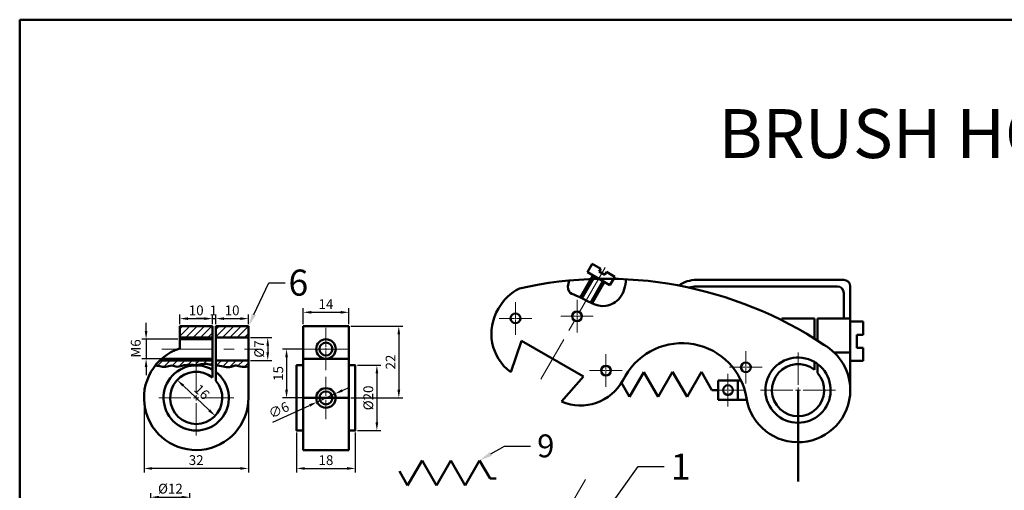
# Model space of a CAD drawing. Units: millimetres. Extents: x 77 to 718, y -35 to 313.
# Tile 3 of 7: x 77 to 379, y 169 to 313. Entities that reach past the tile are written whole.
import ezdxf
from ezdxf import colors
from ezdxf.entities.mleader import LeaderData, LeaderLine
from ezdxf.math import Vec2, Vec3

# ---------------------------------------------------------------- set-up
doc = ezdxf.new("R2010")
doc.units = ezdxf.units.MM
doc.header["$LTSCALE"] = 0.5
doc.linetypes.add('CENTER', pattern=[50.800000000000004, 31.75, -6.349999999999999, 6.349999999999999, -6.349999999999999])
for name, color, linetype, lineweight in [('M-CNTR', 1, 'CENTER', 18), ('M-DIMS', 2, 'Continuous', 25), ('M-HATC', 8, 'Continuous', 18), ('M-OUTL', 7, 'Continuous', 50), ('M-TEXT', 3, 'Continuous', 25)]:
    doc.layers.add(name, color=color, linetype=linetype, lineweight=lineweight)
doc.styles.get("Standard").update_dxf_attribs({"font": 'arial.ttf'})
doc.dimstyles.new('ISO-25', dxfattribs={"dimtxt": 3, "dimasz": 2.5, "dimexe": 1.25, "dimexo": 0.625, "dimtad": 1, "dimtxsty": 'Standard', "dimcen": 2.5, "dimadec": 0, "dimazin": 0, "dimtfac": 1, "dimtmove": 0, "dimatfit": 3, "dimfxl": 1, "dimarcsym": 0})
pattern_1 = [(45, (-102.577664864981, 114.7341887866325), (-1.122532015133644, 1.122532015133644), [])]

# ---------------------------------------------------------------- blocks, each defined once
blk = doc.blocks.new('*D2')
at = {"layer": 'Defpoints', "color": 0, "transparency": 16777216}
for p in [(129.6092219175839, 166.4736375259157), (117.6092219175839, 162.0709279252485), (129.6092219175839, 162.0709279252485)]:
    blk.add_point(p, dxfattribs=at)
at = {"layer": 'M-DIMS', "color": 0, "lineweight": -2, "transparency": 16777216}
for p, q in [((117.6092219175839, 162.6959279252485), (117.6092219175839, 167.7236375259157)), ((120.1092219175839, 166.4736375259157), (127.1092219175839, 166.4736375259157)), ((129.6092219175839, 162.6959279252485), (129.6092219175839, 167.7236375259157))]:
    blk.add_line(p, q, dxfattribs=at)
at = {"layer": 'M-DIMS', "color": 0, "transparency": 16777216}
for points in [[(120.1092219175839, 166.8903041925824), (120.1092219175839, 166.0569708592491), (117.6092219175839, 166.4736375259157)], [(127.1092219175839, 166.8903041925824), (127.1092219175839, 166.0569708592491), (129.6092219175839, 166.4736375259157)]]:
    blk.add_solid(points, dxfattribs=at)
at = {"layer": 'M-DIMS', "color": 0, "transparency": 16777216, "insert": (123.6092219175839, 168.7142582626142), "char_height": 3, "attachment_point": 5}
blk.add_mtext('%%C12', dxfattribs=at)
blk = doc.blocks.new('*U32')
at = {"layer": 'M-CNTR', "color": 0, "transparency": 16777216}
for p, q in [((0, 1.6), (0, 11.5)), ((-11.5, 0), (-1.599999999999999, 0)), ((1.6, 0), (11.5, 0)), ((0, -11.5), (0, -1.599999999999999))]:
    blk.add_line(p, q, dxfattribs=at)
at = {"layer": 'M-CNTR', "color": 0, "linetype": 'Continuous', "transparency": 16777216}
for p, q in [((-0.8, 0), (0.8, 0)), ((0, -0.8), (0, 0.8))]:
    blk.add_line(p, q, dxfattribs=at)
blk = doc.blocks.new('*U33')
at = {"layer": 'M-CNTR', "color": 0, "transparency": 16777216}
for p, q in [((0, 1.6), (0, 11.5)), ((-11.5, 0), (-1.599999999999999, 0)), ((1.6, 0), (11.5, 0)), ((0, -11.5), (0, -1.599999999999999))]:
    blk.add_line(p, q, dxfattribs=at)
at = {"layer": 'M-CNTR', "color": 0, "linetype": 'Continuous', "transparency": 16777216}
for p, q in [((-0.8, 0), (0.8, 0)), ((0, -0.8), (0, 0.8))]:
    blk.add_line(p, q, dxfattribs=at)
blk = doc.blocks.new('*U34')
at = {"layer": 'M-CNTR', "color": 0, "transparency": 16777216}
for p, q in [((0, 0.6000000000000001), (0, 6.5)), ((-6.5, 0), (-0.5999999999999996, 0)), ((0.6000000000000001, 0), (6.5, 0)), ((0, -6.5), (0, -0.5999999999999996))]:
    blk.add_line(p, q, dxfattribs=at)
at = {"layer": 'M-CNTR', "color": 0, "linetype": 'Continuous', "transparency": 16777216}
for p, q in [((-0.3, 0), (0.3, 0)), ((0, -0.3), (0, 0.3))]:
    blk.add_line(p, q, dxfattribs=at)
blk = doc.blocks.new('*U35')
at = {"layer": 'M-CNTR', "color": 0, "transparency": 16777216}
for p, q in [((0, 0.6000000000000001), (0, 6.5)), ((-6.5, 0), (-0.5999999999999996, 0)), ((0.6000000000000001, 0), (6.5, 0)), ((0, -6.5), (0, -0.5999999999999996))]:
    blk.add_line(p, q, dxfattribs=at)
at = {"layer": 'M-CNTR', "color": 0, "linetype": 'Continuous', "transparency": 16777216}
for p, q in [((-0.3, 0), (0.3, 0)), ((0, -0.3), (0, 0.3))]:
    blk.add_line(p, q, dxfattribs=at)
blk = doc.blocks.new('*D36')
at = {"layer": 'Defpoints', "color": 0, "transparency": 16777216}
for p in [(178.2884430352653, 223.1732257711527), (164.2884430352653, 218.9185971032211), (178.2884430352653, 218.9185971032211)]:
    blk.add_point(p, dxfattribs=at)
at = {"layer": 'M-DIMS', "color": 0, "lineweight": -2, "transparency": 16777216}
for p, q in [((164.2884430352653, 219.5435971032211), (164.2884430352653, 224.4232257711527)), ((178.2884430352653, 219.5435971032211), (178.2884430352653, 224.4232257711527)), ((166.7884430352653, 223.1732257711527), (175.7884430352653, 223.1732257711527))]:
    blk.add_line(p, q, dxfattribs=at)
at = {"layer": 'M-DIMS', "color": 0, "transparency": 16777216}
for points in [[(166.7884430352653, 223.5898924378194), (166.7884430352653, 222.7565591044861), (164.2884430352653, 223.1732257711527)], [(175.7884430352653, 223.5898924378194), (175.7884430352653, 222.7565591044861), (178.2884430352653, 223.1732257711527)]]:
    blk.add_solid(points, dxfattribs=at)
at = {"layer": 'M-DIMS', "color": 0, "transparency": 16777216, "insert": (171.2884430352653, 225.3043649253137), "char_height": 3, "attachment_point": 5}
blk.add_mtext('14', dxfattribs=at)
blk = doc.blocks.new('*D37')
at = {"layer": 'Defpoints', "color": 0, "transparency": 16777216}
for p in [(178.2884430352654, 218.9185971032212), (178.2884430352654, 196.9185971032212), (193.6241074583753, 196.9185971032212)]:
    blk.add_point(p, dxfattribs=at)
at = {"layer": 'M-DIMS', "color": 0, "lineweight": -2, "transparency": 16777216}
for p, q in [((178.9134430352654, 218.9185971032212), (194.8741074583753, 218.9185971032213)), ((193.6241074583753, 216.4185971032212), (193.6241074583753, 199.4185971032212)), ((178.9134430352654, 196.9185971032212), (194.8741074583753, 196.9185971032212))]:
    blk.add_line(p, q, dxfattribs=at)
at = {"layer": 'M-DIMS', "color": 0, "transparency": 16777216}
for points in [[(193.2074407917086, 216.4185971032212), (194.0407741250419, 216.4185971032212), (193.6241074583753, 218.9185971032213)], [(193.2074407917086, 199.4185971032212), (194.0407741250419, 199.4185971032212), (193.6241074583753, 196.9185971032212)]]:
    blk.add_solid(points, dxfattribs=at)
at = {"layer": 'M-DIMS', "color": 0, "transparency": 16777216, "insert": (191.4929683042143, 207.918597103221), "char_height": 3, "attachment_point": 5, "rotation": 90}
blk.add_mtext('22', dxfattribs=at)
blk = doc.blocks.new('*D38')
at = {"layer": 'Defpoints', "color": 0, "transparency": 16777216}
for p in [(180.2884430352653, 206.9185971032212), (180.2884430352653, 186.9185971032211), (186.8937752468204, 186.9185971032211)]:
    blk.add_point(p, dxfattribs=at)
at = {"layer": 'M-DIMS', "color": 0, "lineweight": -2, "transparency": 16777216}
for p, q in [((180.9134430352653, 206.9185971032212), (188.1437752468203, 206.9185971032212)), ((186.8937752468203, 204.4185971032212), (186.8937752468204, 189.4185971032211)), ((180.9134430352653, 186.9185971032211), (188.1437752468204, 186.9185971032211))]:
    blk.add_line(p, q, dxfattribs=at)
at = {"layer": 'M-DIMS', "color": 0, "transparency": 16777216}
for points in [[(186.4771085801537, 204.4185971032212), (187.310441913487, 204.4185971032212), (186.8937752468203, 206.9185971032212)], [(186.4771085801537, 189.4185971032211), (187.310441913487, 189.4185971032211), (186.8937752468204, 186.9185971032211)]]:
    blk.add_solid(points, dxfattribs=at)
at = {"layer": 'M-DIMS', "color": 0, "transparency": 16777216, "insert": (184.6531545101218, 196.9185971032211), "char_height": 3, "attachment_point": 5, "rotation": 90}
blk.add_mtext('%%C20', dxfattribs=at)
blk = doc.blocks.new('*D39')
at = {"layer": 'Defpoints', "color": 0, "transparency": 16777216}
for p in [(136.5191626098565, 221.2361377014674), (126.5191626098565, 218.9185971032211), (136.5191626098565, 218.9185971032211)]:
    blk.add_point(p, dxfattribs=at)
at = {"layer": 'M-DIMS', "color": 0, "lineweight": -2, "transparency": 16777216}
for p, q in [((126.5191626098565, 219.5435971032211), (126.5191626098565, 222.4861377014674)), ((129.0191626098565, 221.2361377014674), (134.0191626098565, 221.2361377014674)), ((136.5191626098565, 219.5435971032211), (136.5191626098565, 222.4861377014674))]:
    blk.add_line(p, q, dxfattribs=at)
at = {"layer": 'M-DIMS', "color": 0, "transparency": 16777216}
for points in [[(129.0191626098565, 221.6528043681341), (129.0191626098565, 220.8194710348007), (126.5191626098565, 221.2361377014674)], [(134.0191626098565, 221.6528043681341), (134.0191626098565, 220.8194710348007), (136.5191626098565, 221.2361377014674)]]:
    blk.add_solid(points, dxfattribs=at)
at = {"layer": 'M-DIMS', "color": 0, "transparency": 16777216, "insert": (131.5191626098565, 223.3928566646325), "char_height": 3, "attachment_point": 5}
blk.add_mtext('10', dxfattribs=at)
blk = doc.blocks.new('*D40')
at = {"layer": 'Defpoints', "color": 0, "transparency": 16777216}
for p in [(137.5191626098565, 221.2361377014674), (136.5191626098565, 218.9185971032211), (137.5191626098565, 218.9185971032211)]:
    blk.add_point(p, dxfattribs=at)
at = {"layer": 'M-DIMS', "color": 0, "lineweight": -2, "transparency": 16777216}
for p, q in [((134.0191626098565, 221.2361377014674), (131.5191626098565, 221.2361377014674)), ((136.5191626098565, 219.5435971032211), (136.5191626098565, 222.4861377014674)), ((136.5191626098565, 221.2361377014674), (137.5191626098565, 221.2361377014674)), ((137.5191626098565, 219.5435971032211), (137.5191626098565, 222.4861377014674)), ((140.0191626098565, 221.2361377014674), (142.5191626098565, 221.2361377014674))]:
    blk.add_line(p, q, dxfattribs=at)
at = {"layer": 'M-DIMS', "color": 0, "transparency": 16777216}
for points in [[(134.0191626098565, 221.6528043681341), (134.0191626098565, 220.8194710348007), (136.5191626098565, 221.2361377014674)], [(140.0191626098565, 221.6528043681341), (140.0191626098565, 220.8194710348007), (137.5191626098565, 221.2361377014674)]]:
    blk.add_solid(points, dxfattribs=at)
at = {"layer": 'M-DIMS', "color": 0, "transparency": 16777216, "insert": (136.7740427016174, 223.3672768556283), "char_height": 3, "attachment_point": 5}
blk.add_mtext('1', dxfattribs=at)
blk = doc.blocks.new('*D41')
at = {"layer": 'Defpoints', "color": 0, "transparency": 16777216}
for p in [(147.5191626098565, 221.2361377014674), (137.5191626098565, 218.9185971032211), (147.5191626098565, 218.9185971032211)]:
    blk.add_point(p, dxfattribs=at)
at = {"layer": 'M-DIMS', "color": 0, "lineweight": -2, "transparency": 16777216}
for p, q in [((137.5191626098565, 219.5435971032211), (137.5191626098565, 222.4861377014674)), ((140.0191626098565, 221.2361377014674), (145.0191626098565, 221.2361377014674)), ((147.5191626098565, 219.5435971032211), (147.5191626098565, 222.4861377014674))]:
    blk.add_line(p, q, dxfattribs=at)
at = {"layer": 'M-DIMS', "color": 0, "transparency": 16777216}
for points in [[(140.0191626098565, 221.6528043681341), (140.0191626098565, 220.8194710348007), (137.5191626098565, 221.2361377014674)], [(145.0191626098565, 221.6528043681341), (145.0191626098565, 220.8194710348007), (147.5191626098565, 221.2361377014674)]]:
    blk.add_solid(points, dxfattribs=at)
at = {"layer": 'M-DIMS', "color": 0, "transparency": 16777216, "insert": (142.5191626098565, 223.3928566646325), "char_height": 3, "attachment_point": 5}
blk.add_mtext('10', dxfattribs=at)
blk = doc.blocks.new('*D42')
at = {"layer": 'Defpoints', "color": 0, "transparency": 16777216}
for p in [(147.5191626098566, 215.4185971032212), (147.5191626098566, 208.4185971032212), (153.4383000049706, 208.4185971032212)]:
    blk.add_point(p, dxfattribs=at)
at = {"layer": 'M-DIMS', "color": 0, "lineweight": -2, "transparency": 16777216}
for p, q in [((148.1441626098566, 215.4185971032212), (154.6883000049706, 215.4185971032212)), ((153.4383000049706, 212.9185971032212), (153.4383000049706, 210.9185971032212)), ((148.1441626098566, 208.4185971032212), (154.6883000049706, 208.4185971032212))]:
    blk.add_line(p, q, dxfattribs=at)
at = {"layer": 'M-DIMS', "color": 0, "transparency": 16777216}
for points in [[(153.0216333383039, 212.9185971032212), (153.8549666716372, 212.9185971032212), (153.4383000049706, 215.4185971032212)], [(153.0216333383039, 210.9185971032212), (153.8549666716372, 210.9185971032212), (153.4383000049706, 208.4185971032212)]]:
    blk.add_solid(points, dxfattribs=at)
at = {"layer": 'M-DIMS', "color": 0, "transparency": 16777216, "insert": (151.1976792682721, 211.9185971032211), "char_height": 3, "attachment_point": 5, "rotation": 90}
blk.add_mtext('%%C7', dxfattribs=at)
blk = doc.blocks.new('*D43')
at = {"layer": 'Defpoints', "color": 0, "transparency": 16777216}
for p in [(126.5191626098566, 214.9185971032212), (116.1550390454235, 208.9185971032212), (126.5191626098566, 208.9185971032212)]:
    blk.add_point(p, dxfattribs=at)
at = {"layer": 'M-DIMS', "color": 0, "lineweight": -2, "transparency": 16777216}
for p, q in [((116.1550390454235, 217.4185971032212), (116.1550390454235, 219.9185971032212)), ((125.8941626098565, 214.9185971032212), (114.9050390454235, 214.9185971032212)), ((116.1550390454235, 214.9185971032212), (116.1550390454235, 208.9185971032212)), ((125.8941626098565, 208.9185971032212), (114.9050390454235, 208.9185971032212)), ((116.1550390454235, 206.4185971032212), (116.1550390454235, 203.9185971032212))]:
    blk.add_line(p, q, dxfattribs=at)
at = {"layer": 'M-DIMS', "color": 0, "transparency": 16777216}
for points in [[(115.7383723787568, 217.4185971032212), (116.5717057120902, 217.4185971032212), (116.1550390454235, 214.9185971032212)], [(115.7383723787568, 206.4185971032212), (116.5717057120902, 206.4185971032212), (116.1550390454235, 208.9185971032212)]]:
    blk.add_solid(points, dxfattribs=at)
at = {"layer": 'M-DIMS', "color": 0, "transparency": 16777216, "insert": (113.3727995653948, 212.0977955691644), "char_height": 3, "attachment_point": 5, "rotation": 90}
blk.add_mtext('M6', dxfattribs=at)
blk = doc.blocks.new('*D44')
at = {"layer": 'Defpoints', "color": 0, "transparency": 16777216}
for p in [(125.713031027325, 202.4221265204524), (137.3252941923879, 191.4150676859897), (137.325294192388, 191.4150676859898)]:
    blk.add_point(p, dxfattribs=at)
at = {"layer": 'M-DIMS', "color": 0, "lineweight": -2, "transparency": 16777216}
for p, q in [((126.1429942630462, 202.8757305503377), (126.5729574987675, 203.329334580223)), ((127.5274471468661, 200.7022735775677), (135.5108780728469, 193.1349206288746)), ((137.7552574281092, 191.868671715875), (138.1852206638304, 192.3222757457603))]:
    blk.add_line(p, q, dxfattribs=at)
at = {"layer": 'M-DIMS', "color": 0, "transparency": 16777216}
for points in [[(127.8140893040136, 201.0046762641578), (127.2408049897187, 200.3998708909775), (125.713031027325, 202.4221265204524)], [(135.7975202299944, 193.4373233154648), (135.2242359156994, 192.8325179422844), (137.325294192388, 191.4150676859898)]]:
    blk.add_solid(points, dxfattribs=at)
at = {"layer": 'M-DIMS', "color": 0, "transparency": 16777216, "insert": (133.0028583921665, 198.4838713640558), "char_height": 3, "attachment_point": 5, "rotation": 316.5326446484607}
blk.add_mtext('16', dxfattribs=at)
blk = doc.blocks.new('*D45')
at = {"layer": 'Defpoints', "color": 0, "transparency": 16777216}
for p in [(115.5191626098565, 196.918597103221), (147.5191626098565, 196.918597103221), (115.5191626098565, 175.3007429935038)]:
    blk.add_point(p, dxfattribs=at)
at = {"layer": 'M-DIMS', "color": 0, "lineweight": -2, "transparency": 16777216}
for p, q in [((115.5191626098565, 196.2935971032211), (115.5191626098565, 174.0507429935038)), ((147.5191626098565, 196.2935971032211), (147.5191626098565, 174.0507429935038)), ((145.0191626098565, 175.3007429935038), (118.0191626098565, 175.3007429935038))]:
    blk.add_line(p, q, dxfattribs=at)
at = {"layer": 'M-DIMS', "color": 0, "transparency": 16777216}
for points in [[(118.0191626098565, 175.7174096601705), (118.0191626098565, 174.8840763268372), (115.5191626098565, 175.3007429935038)], [(145.0191626098565, 175.7174096601705), (145.0191626098565, 174.8840763268372), (147.5191626098565, 175.3007429935038)]]:
    blk.add_solid(points, dxfattribs=at)
at = {"layer": 'M-DIMS', "color": 0, "transparency": 16777216, "insert": (131.5191626098565, 177.458485149029), "char_height": 3, "attachment_point": 5}
blk.add_mtext('32', dxfattribs=at)
blk = doc.blocks.new('*D46')
at = {"layer": 'Defpoints', "color": 0, "transparency": 16777216}
for p in [(162.2884430352654, 186.9185971032211), (180.2884430352653, 186.9185971032211), (180.2884430352653, 175.3007429935038)]:
    blk.add_point(p, dxfattribs=at)
at = {"layer": 'M-DIMS', "color": 0, "lineweight": -2, "transparency": 16777216}
for p, q in [((162.2884430352654, 186.2935971032211), (162.2884430352654, 174.0507429935038)), ((180.2884430352653, 186.2935971032211), (180.2884430352653, 174.0507429935038)), ((164.7884430352654, 175.3007429935038), (177.7884430352653, 175.3007429935038))]:
    blk.add_line(p, q, dxfattribs=at)
at = {"layer": 'M-DIMS', "color": 0, "transparency": 16777216}
for points in [[(164.7884430352654, 175.7174096601705), (164.7884430352654, 174.8840763268372), (162.2884430352654, 175.3007429935038)], [(177.7884430352653, 175.7174096601705), (177.7884430352653, 174.8840763268372), (180.2884430352653, 175.3007429935038)]]:
    blk.add_solid(points, dxfattribs=at)
at = {"layer": 'M-DIMS', "color": 0, "transparency": 16777216, "insert": (171.2884430352653, 177.4574619566689), "char_height": 3, "attachment_point": 5}
blk.add_mtext('18', dxfattribs=at)
blk = doc.blocks.new('*D47')
at = {"layer": 'Defpoints', "color": 0, "transparency": 16777216}
for p in [(164.7884430352654, 211.9185971032212), (159.2157581517809, 196.9185971032212), (164.7884430352654, 196.9185971032212)]:
    blk.add_point(p, dxfattribs=at)
at = {"layer": 'M-DIMS', "color": 0, "lineweight": -2, "transparency": 16777216}
for p, q in [((164.1634430352654, 211.9185971032212), (157.9657581517809, 211.9185971032212)), ((159.2157581517809, 209.4185971032212), (159.2157581517809, 199.4185971032212)), ((164.1634430352654, 196.9185971032212), (157.9657581517809, 196.9185971032212))]:
    blk.add_line(p, q, dxfattribs=at)
at = {"layer": 'M-DIMS', "color": 0, "transparency": 16777216}
for points in [[(158.7990914851142, 209.4185971032212), (159.6324248184475, 209.4185971032212), (159.2157581517809, 211.9185971032212)], [(158.7990914851142, 199.4185971032212), (159.6324248184475, 199.4185971032212), (159.2157581517809, 196.9185971032212)]]:
    blk.add_solid(points, dxfattribs=at)
at = {"layer": 'M-DIMS', "color": 0, "transparency": 16777216, "insert": (157.0590391886158, 204.4185971032211), "char_height": 3, "attachment_point": 5, "rotation": 90}
blk.add_mtext('15', dxfattribs=at)
blk = doc.blocks.new('*D48')
at = {"layer": 'Defpoints', "color": 0, "transparency": 16777216}
for p in [(174.0172356011557, 198.1650685759558), (168.559650469375, 195.6721256304863)]:
    blk.add_point(p, dxfattribs=at)
at = {"layer": 'M-DIMS', "color": 0, "lineweight": -2, "transparency": 16777216}
for p, q in [((176.2912294060643, 199.2037948032348), (178.565223210973, 200.2425210305137)), ((174.0172356011557, 198.1650685759558), (168.559650469375, 195.6721256304863)), ((154.9824047553545, 189.4702436434197), (166.2856566644664, 194.6333994032073))]:
    blk.add_line(p, q, dxfattribs=at)
at = {"layer": 'M-DIMS', "color": 0, "transparency": 16777216}
for points in [[(176.1181083681845, 199.5827937707196), (176.4643504439441, 198.82479583575), (174.0172356011557, 198.1650685759558)], [(166.1125356265865, 195.0123983706921), (166.4587777023462, 194.2544004357225), (168.559650469375, 195.6721256304863)]]:
    blk.add_solid(points, dxfattribs=at)
at = {"layer": 'M-DIMS', "color": 0, "transparency": 16777216, "insert": (156.9978678129276, 192.854186978335), "char_height": 3, "attachment_point": 5, "rotation": 24.550208828109366}
blk.add_mtext('∅6', dxfattribs=at)
blk = doc.blocks.new('*U119')
at = {"layer": 'M-CNTR', "color": 0, "transparency": 16777216}
for p, q in [((0, 0.3), (0, 5)), ((-5, 0), (-0.2999999999999998, 0)), ((0.3, 0), (5, 0)), ((0, -5), (0, -0.2999999999999998))]:
    blk.add_line(p, q, dxfattribs=at)
at = {"layer": 'M-CNTR', "color": 0, "linetype": 'Continuous', "transparency": 16777216}
for p, q in [((-0.15, 0), (0.15, 0)), ((0, -0.15), (0, 0.15))]:
    blk.add_line(p, q, dxfattribs=at)
blk = doc.blocks.new('*U120')
at = {"layer": 'M-CNTR', "color": 0, "transparency": 16777216}
for p, q in [((0, 0.3), (0, 5)), ((-5, 0), (-0.2999999999999998, 0)), ((0.3, 0), (5, 0)), ((0, -5), (0, -0.2999999999999998))]:
    blk.add_line(p, q, dxfattribs=at)
at = {"layer": 'M-CNTR', "color": 0, "linetype": 'Continuous', "transparency": 16777216}
for p, q in [((-0.15, 0), (0.15, 0)), ((0, -0.15), (0, 0.15))]:
    blk.add_line(p, q, dxfattribs=at)
blk = doc.blocks.new('*U121')
at = {"layer": 'M-CNTR', "color": 0, "transparency": 16777216}
for p, q in [((0, 0.3), (0, 5)), ((-5, 0), (-0.2999999999999998, 0)), ((0.3, 0), (5, 0)), ((0, -5), (0, -0.2999999999999998))]:
    blk.add_line(p, q, dxfattribs=at)
at = {"layer": 'M-CNTR', "color": 0, "linetype": 'Continuous', "transparency": 16777216}
for p, q in [((-0.15, 0), (0.15, 0)), ((0, -0.15), (0, 0.15))]:
    blk.add_line(p, q, dxfattribs=at)
blk = doc.blocks.new('*U122')
at = {"layer": 'M-CNTR', "color": 0, "transparency": 16777216}
for p, q in [((0, 0.3), (0, 5)), ((-5, 0), (-0.2999999999999998, 0)), ((0.3, 0), (5, 0)), ((0, -5), (0, -0.2999999999999998))]:
    blk.add_line(p, q, dxfattribs=at)
at = {"layer": 'M-CNTR', "color": 0, "linetype": 'Continuous', "transparency": 16777216}
for p, q in [((-0.15, 0), (0.15, 0)), ((0, -0.15), (0, 0.15))]:
    blk.add_line(p, q, dxfattribs=at)
blk = doc.blocks.new('*U123')
at = {"layer": 'M-CNTR', "color": 0, "transparency": 16777216}
for p, q in [((0, 0.3), (0, 5)), ((-5, 0), (-0.2999999999999998, 0)), ((0.3, 0), (5, 0)), ((0, -5), (0, -0.2999999999999998))]:
    blk.add_line(p, q, dxfattribs=at)
at = {"layer": 'M-CNTR', "color": 0, "linetype": 'Continuous', "transparency": 16777216}
for p, q in [((-0.15, 0), (0.15, 0)), ((0, -0.15), (0, 0.15))]:
    blk.add_line(p, q, dxfattribs=at)

msp = doc.modelspace()

# ---------------------------------------------------------------- hatches: boundary and pattern name
at = {"layer": 'M-HATC'}
h = msp.add_hatch(dxfattribs=at)
h.set_pattern_fill('ANSI31', color=256, scale=0.5)
h.set_pattern_definition(pattern_1)
h.paths.add_polyline_path([(126.5191626098565, 218.9185971032211), (126.5191626098565, 215.4185971032211), (136.5191626098565, 215.4185971032211), (136.5191626098565, 218.9185971032211)])
h.paths.add_polyline_path([(147.5191626098565, 215.4185971032211), (147.5191626098565, 218.9185971032211), (137.5191626098565, 218.9185971032211), (137.5191626098565, 215.4185971032211)])
edge = h.paths.add_edge_path()
edge.add_spline(control_points=[(118.9557939554484, 206.8262591913949), (119.1622428321333, 206.8207418574951), (119.9060149552565, 206.8008645919243), (120.9256160174756, 206.4639081365), (122.4285901625097, 206.4493117959326), (123.9320579436518, 207.1043540555595), (125.8288620433754, 206.1876524210258), (128.280696105137, 207.2913325437914), (130.2297108814224, 207.0704143910512), (131.4713748263492, 206.9242252610243)], knot_values=[0.0474336215315763, 0.0474336215315763, 0.0474336215315763, 0.0474336215315763, 0.665543400871659, 2.274293996290248, 3.218093393399181, 5.13413874826128, 6.892654807734232, 9.00059992640355, 12.69799411755507, 12.69799411755507, 12.69799411755507, 12.69799411755507], degree=3, periodic=0)
edge.add_spline(control_points=[(136.5191626098565, 207.0370106034905), (135.9002037074706, 207.1304193094326), (134.2456568584692, 207.5440129440283), (132.5725553613335, 207.1746715013177), (131.5191626098565, 206.9350974611666)], knot_values=[0.0741311551398187, 0.0741311551398267, 0.0741311551398267, 0.0741311551398267, 1.944637449859328, 5.122794371168017, 5.122794371168017, 5.122794371168017, 5.122794371168017], degree=3, periodic=0)
edge.add_line((131.5191626098565, 206.9350974611666), (131.5191626098565, 208.4185971032211))
edge.add_line((131.5191626098565, 208.4185971032211), (120.394864879213, 208.4185971032211))
edge.add_arc((131.5191626098565, 196.9185971032211), 15.99999999999999, 134.0486256740844, 141.7401549148765)
edge = h.paths.add_edge_path()
edge.add_spline(control_points=[(137.5191626098565, 206.9179853636143), (137.7259563826982, 206.8956881364361), (138.6658059260099, 206.7888454592824), (140.1956370481373, 206.4009850892262), (142.0509265619373, 206.2030664292616), (143.514512736489, 207.0528617066396), (145.2971958708007, 206.296980285455), (146.6698495489315, 206.4476098349519), (147.5191626098565, 206.5408100687669)], knot_values=[6.128080963507823, 6.128080963507823, 6.128080963507823, 6.128080963507823, 6.752419313148968, 8.97305734251825, 10.89473593504874, 12.14514412431177, 13.71387867391477, 16.25972873465652, 16.25972873465652, 16.25972873465652, 16.25972873465652], degree=3, periodic=0)
edge.add_line((147.5191626098565, 206.5408100687669), (147.5191626098565, 208.4185971032211))
edge.add_line((147.5191626098565, 208.4185971032211), (137.5191626098565, 208.4185971032211))
edge.add_line((137.5191626098565, 208.4185971032211), (137.5191626098565, 206.9179853636143))
h = msp.add_hatch(dxfattribs=at)
h.set_pattern_fill('ANSI31', color=256, scale=0.5)
h.set_pattern_definition(pattern_1)
edge = h.paths.add_edge_path()
edge.add_line((131.5191626098565, 208.4185971032211), (131.5191626098565, 206.9350974611666))
edge.add_spline(control_points=[(131.5191626098565, 206.9350974611666), (132.5725553613335, 207.1746715013177), (134.2456568584692, 207.5440129440283), (135.9002037074706, 207.1304193094326), (136.5191626098565, 207.0370106034905)], knot_values=[0.0741311551398185, 0.0741311551398185, 0.0741311551398185, 0.0741311551398185, 3.252288076448508, 5.122794371168009, 5.122794371168009, 5.122794371168009, 5.122794371168017], degree=3, periodic=0)
edge.add_line((136.5191626098565, 207.0370106034905), (136.5191626098565, 208.4185971032211))
edge.add_line((136.5191626098565, 208.4185971032211), (131.5191626098565, 208.4185971032211))

# ---------------------------------------------------------------- linework, layer by layer
at = {"layer": 'M-CNTR'}
for p, q in [((256.852973873791, 236.8845362904707), (237.1241646983158, 202.7132364257164)), ((120.9511040420905, 211.9185971032211), (150.8393795507288, 211.9185971032211)), ((164.2884430352653, 211.9185971032211), (178.2884430352653, 211.9185971032211)), ((250.8010208058587, 171.9409756890816), (206.6822855769689, 95.52508470696544))]:
    msp.add_line(p, q, dxfattribs=at)
at = {"layer": 'M-OUTL'}
for p, q in [((252.9061685986866, 238.0484690264091), (251.4061685986866, 235.4503928150557)), ((251.4061685986866, 235.4503928150557), (258.3343718289622, 231.4503928150557)), ((255.50424481004, 236.5484690264091), (252.9061685986866, 238.0484690264091)), ((255.0042448100399, 235.6824436226246), (255.50424481004, 236.5484690264091)), ((256.7362956176089, 234.6824436226246), (255.0042448100399, 235.6824436226246)), ((257.2362956176089, 235.5484690264091), (256.7362956176089, 234.6824436226246)), ((259.8343718289622, 234.0484690264091), (257.2362956176089, 235.5484690264091)), ((249.2504351402668, 227.7165529374964), (253.1382194062555, 234.4503928150557)), ((256.6023210213933, 232.4503928150557), (252.8288835307475, 225.914607362072)), ((258.3343718289622, 231.4503928150557), (259.8343718289622, 234.0484690264091)), ((320.9872440844801, 221.3080967638909), (310.9872440844802, 221.3080967638909)), ((310.9872440844802, 221.3080967638909), (310.9872440844802, 220.7305792519626)), ((320.9872440844801, 221.3080967638909), (320.9872440844801, 215.0995571999182)), ((331.9872440844802, 221.3080967638909), (321.9872440844802, 221.3080967638909)), ((321.9872440844802, 221.3080967638909), (321.9872440844802, 214.4647525200195)), ((331.9872440844802, 199.3080967638909), (331.9872440844802, 221.3080967638909)), ((335.9872440844802, 220.3080967638909), (331.9872440844802, 220.3080967638909)), ((331.9872440844802, 220.3080967638909), (331.9872440844802, 208.3080967638909)), ((335.9872440844802, 216.3080967638909), (335.9872440844802, 220.3080967638909)), ((126.5191626098565, 218.9185971032211), (126.5191626098565, 212.1172812567917)), ((136.5191626098565, 218.9185971032211), (126.5191626098565, 218.9185971032211)), ((136.5191626098565, 218.9185971032211), (136.5191626098565, 203.1635951016195)), ((147.5191626098565, 218.9185971032211), (137.5191626098565, 218.9185971032211)), ((137.5191626098565, 218.9185971032211), (137.5191626098565, 202.2100997253503)), ((147.5191626098565, 196.918597103221), (147.5191626098565, 218.9185971032211)), ((164.2884430352653, 218.9185971032211), (178.2884430352653, 218.9185971032211)), ((164.2884430352653, 218.9185971032211), (164.2884430352653, 180.9185971032211)), ((178.2884430352653, 218.9185971032211), (178.2884430352653, 180.9185971032211)), ((136.5191626098565, 214.9185971032211), (126.5191626098565, 214.9185971032211)), ((137.5191626098565, 215.4185971032211), (147.5191626098565, 215.4185971032211)), ((227.9468815325274, 204.8177157071243), (231.2148307249584, 214.4779697449687)), ((231.2148307249584, 214.4779697449687), (250.2673896082161, 203.4779697449687)), ((333.9872440844802, 212.3080967638909), (333.9872440844802, 216.3080967638909)), ((333.9872440844802, 216.3080967638909), (335.9872440844802, 216.3080967638909)), ((335.9872440844802, 212.3080967638909), (333.9872440844802, 212.3080967638909)), ((335.9872440844802, 208.3080967638909), (335.9872440844802, 212.3080967638909)), ((136.5191626098565, 208.9185971032211), (120.9361573655981, 208.9185971032211)), ((137.5191626098565, 208.4185971032211), (147.5191626098565, 208.4185971032211)), ((164.2884430352653, 208.9185971032211), (178.2884430352653, 208.9185971032211)), ((327.1115418151236, 210.8080967638909), (331.9872440844802, 210.8080967638909)), ((331.9872440844802, 208.3080967638909), (335.9872440844802, 208.3080967638909)), ((320.9872440844801, 207.9683508017353), (320.9872440844801, 205.5530947622894)), ((321.9872440844802, 207.3080967638909), (321.9872440844802, 204.5995993860201)), ((243.5353388006472, 195.8177157071243), (250.2673896082161, 203.4779697449687)), ((263.1043162038423, 203.7121788216254), (261.8558653614581, 201.549798531864)), ((264.3447372881748, 197.2389459012589), (268.740227913197, 204.8521589879901)), ((268.740227913197, 204.8521589879901), (273.1357185382192, 197.2389459012589)), ((273.1357185382192, 197.2389459012589), (277.5503436051493, 204.8853008135491)), ((277.5503436051493, 204.8853008135491), (281.9649686720794, 197.2389459012589)), ((281.9649686720794, 197.2389459012589), (286.3795937390094, 204.8853008135491)), ((286.3795937390094, 204.8853008135491), (289.5995939984052, 199.3080967638909)), ((291.5155357290359, 202.3080967638909), (298.4833456677799, 202.3080967638909)), ((291.5155357290359, 196.3080967638909), (291.5155357290359, 202.3080967638909)), ((297.5155357290359, 196.3080967638909), (297.5155357290359, 202.3080967638909)), ((261.8558653614581, 201.549798531864), (264.3447372881748, 197.2389459012589)), ((289.5995939984052, 199.3080967638909), (291.5155357290359, 199.3080967638909)), ((315.9872440844802, 199.3080967638909), (315.9872440844802, 171.3080967638909)), ((164.2884430352653, 196.918597103221), (178.2884430352653, 196.918597103221)), ((300.2710104389785, 196.3080967638909), (291.5155357290359, 196.3080967638909)), ((164.2884430352653, 180.9185971032211), (178.2884430352653, 180.9185971032211)), ((196.3323562524466, 170.1084467105109), (200.7278468774688, 177.7216597972421)), ((200.7278468774688, 177.7216597972421), (205.123337502491, 170.1084467105109)), ((205.123337502491, 170.1084467105109), (209.5379625694211, 177.7548016228011)), ((209.5379625694211, 177.7548016228011), (213.9525876363513, 170.1084467105109)), ((213.9525876363513, 170.1084467105109), (218.3672127032813, 177.7548016228011)), ((218.3672127032813, 177.7548016228011), (221.587212962677, 172.1775975731429)), ((193.84348432573, 174.419299341116), (196.3323562524466, 170.1084467105109)), ((221.587212962677, 172.1775975731429), (223.5031546933078, 172.1775975731429))]:
    msp.add_line(p, q, dxfattribs=at)
at = {"layer": 'M-OUTL', "transparency": 33554559}
for p, q in [((249.6973953695372, 227.4907107635554), (253.5712321081478, 234.2003928150557)), ((256.169308319501, 232.7003928150557), (252.3720349626665, 226.1233224307907)), ((136.5191626098565, 215.4185971032211), (126.5191626098565, 215.4185971032211)), ((136.5191626098565, 208.4185971032211), (120.394864879213, 208.4185971032211))]:
    msp.add_line(p, q, dxfattribs=at)
at = {"layer": 'M-OUTL', "ltscale": 0.5}
for p, q in [((326.8886615455381, 233.1237524903359), (329.9872440844802, 233.1237524903359)), ((331.9872440844802, 220.3080967638909), (331.9872440844802, 231.1237524903359))]:
    msp.add_line(p, q, dxfattribs=at)
msp.add_lwpolyline([(77.41772587536796, 312.9124059195133), (718.0121353131708, 312.9124059195133), (718.0121353131708, -34.89770349051241), (77.41772587536796, -34.89770349051241)], close=True, dxfattribs=at)
for points in [[(279.420987962987, 231.3925712933891, -0.1545301937118154), (284.8886615455381, 233.1237524903359), (326.8886615455381, 233.1237524903359)], [(282.5670462525224, 230.7553794036872, -0.0788423554792563), (284.8886615455381, 231.1237524903359), (327.9872440844802, 231.1237524903359, -0.4142135623730951), (329.9872440844802, 229.1237524903359), (329.9872440844802, 221.3080967638909)]]:
    msp.add_lwpolyline(points, format="xyb", dxfattribs=at)
at = {"layer": 'M-OUTL'}
for points in [[(164.2884430352654, 206.9185971032211), (162.2884430352654, 206.9185971032211), (162.2884430352654, 186.9185971032211), (164.2884430352654, 186.9185971032211)], [(178.2884430352653, 206.9185971032211), (180.2884430352653, 206.9185971032211), (180.2884430352653, 186.9185971032211), (178.2884430352653, 186.9185971032211)]]:
    msp.add_lwpolyline(points, dxfattribs=at)
for centre, radius in [((248.2411101665873, 221.9683508017353), 1.5), ((229.3847037060363, 221.308096763891), 1.5), ((171.2884430352653, 211.9185971032211), 3), ((171.2884430352653, 211.9185971032211), 2.000000000000006), ((257.0975166271384, 205.3080967638909), 1.5), ((299.9872440844801, 206.3080967638909), 1.5), ((171.2884430352653, 196.918597103221), 3), ((294.515535729036, 199.3080967638909), 1.5), ((171.2884430352653, 196.918597103221), 2.000000000000006)]:
    msp.add_circle(centre, radius, dxfattribs=at)
for centre, radius, start, end in [((257.1754235371662, 113.4725354072994), 120, 56.23567770499765, 102.8097892519008), ((237.093589112549, 217.3629018539724), 14.655228886317, 116.4338216500028, 151.7118829249539), ((236.6557854241631, 216.604603621947), 14.655228886317, 148.2881170750466, 233.5406493650028), ((131.5191626098565, 196.918597103221), 16, 108.209956864283, 0), ((280.4248242795311, 193.7121788216254), 20, 8.942441268981947, 149.9999999999994), ((315.9872440844802, 199.3080967638909), 16, 0, 60.48860419314383), ((315.9872440844802, 199.3080967638909), 10, 60.00000000000028, 53.13010235415434), ((131.5191626098565, 196.918597103221), 10, 59.99999999999986, 53.13010235415614), ((315.9872440844802, 199.3080967638909), 8, 51.31781254651103, 41.40962210927096), ((315.9872440844802, 199.3080967638909), 10, 53.13010235415532, 60.00000000000028), ((131.5191626098565, 196.918597103221), 8, 51.31781254651052, 41.40962210927096), ((249.3886312206256, 209.2532916738094), 14.655228886317, 246.4593506349944, 331.7118829249539), ((315.9872440844802, 199.3080967638909), 16, 188.9424412689819, 0)]:
    msp.add_arc(centre, radius, start, end, dxfattribs=at)
at = {"layer": 'M-OUTL', "ltscale": 0.5}
msp.add_arc((329.9872440844802, 231.1237524903359), 2, 0, 90, dxfattribs=at)
at = {"layer": 'M-OUTL'}
for points, knots in [([(245.8017736647339, 232.9323198059803), (245.5133538125845, 231.6357068684466), (245.0181149932678, 229.4093238524728), (250.5194602516519, 227.5017717520864), (255.3798465541132, 223.5051990759465), (262.344827095545, 227.4805838907594), (262.9831190576604, 231.2461478043164), (263.3337058237765, 233.3144127260332)], [0, 0, 0, 0, 3.376490024437771, 5.797690140522398, 15.51431558055696, 20.46882088574361, 26.50619531207646, 26.50619531207646, 26.50619531207646, 26.50619531207646]), ([(131.5191626098565, 206.9185971032211), (130.2615649549577, 207.0667329839094), (128.2960717784234, 207.2982538217216), (125.8288620433754, 206.1876524210258), (123.9320579436518, 207.1043540555595), (122.4285901625096, 206.4493117959326), (120.9256160174757, 206.4639081365), (119.9060149552565, 206.8008645919243), (119.1622428321333, 206.8207418574951), (118.9557939554484, 206.8262591913949)], [0, 0, 0, 0, 3.744827812683098, 5.852772931352416, 7.611288990825368, 9.527334345687468, 10.4711337427964, 12.07988433821499, 12.69799411755507, 12.69799411755507, 12.69799411755507, 12.69799411755507]), ([(131.4454506284043, 206.9183254267202), (132.5234179799587, 207.1636563807687), (134.2213626118734, 207.5500858731542), (135.9002037074706, 207.1304193094326), (136.5191626098565, 207.0370106034905)], [0, 0, 0, 0, 3.252288076448508, 5.122794371168009, 5.122794371168009, 5.122794371168009, 5.122794371168017]), ([(137.5191626098565, 206.9179853636143), (137.7259563826982, 206.8956881364361), (138.6658059260099, 206.7888454592824), (140.1956370481373, 206.4009850892262), (142.0509265619373, 206.2030664292616), (143.514512736489, 207.0528617066396), (145.2971958708007, 206.296980285455), (146.6698495489315, 206.4476098349519), (147.5191626098565, 206.5408100687669)], [6.128080963507823, 6.128080963507823, 6.128080963507823, 6.128080963507823, 6.752419313148968, 8.97305734251825, 10.89473593504874, 12.14514412431177, 13.71387867391477, 16.25972873465652, 16.25972873465652, 16.25972873465652, 16.25972873465652])]:
    msp.add_open_spline(points, degree=3, knots=knots, dxfattribs=at)

# ---------------------------------------------------------------- block references
at = {"layer": 'M-CNTR'}
for name, p in [('*U123', (248.2411101665873, 221.9683508017353)), ('*U122', (229.3847037060363, 221.308096763891)), ('*U34', (171.2884430352653, 211.9185971032211)), ('*U119', (299.9872440844801, 206.3080967638909)), ('*U32', (131.5191626098565, 196.918597103221)), ('*U121', (257.0975166271384, 205.3080967638909)), ('*U33', (315.9872440844802, 199.3080967638909)), ('*U35', (171.2884430352653, 196.918597103221)), ('*U120', (294.515535729036, 199.3080967638909))]:
    msp.add_blockref(name, p, dxfattribs=at)

# ---------------------------------------------------------------- texts
at = {"layer": 'M-TEXT', "ltscale": 0.5, "insert": (291.6413907524809, 285.4817069065082), "char_height": 15, "attachment_point": 1}
msp.add_mtext_dynamic_manual_height_columns('BRUSH HOLDER', width=204.6504499458852, gutter_width=12.5, heights=[0], dxfattribs=at)

# ---------------------------------------------------------------- dimensions: what is measured, and where the dimension line sits
at = {"layer": 'M-DIMS'}
for base, p1, p2, picture, middle in [((178.2884430352653, 223.1732257711527), (164.2884430352653, 218.9185971032211), (178.2884430352653, 218.9185971032211), '*D36', (171.2884430352653, 225.3043649253137)), ((136.5191626098565, 221.2361377014674), (126.5191626098565, 218.9185971032211), (136.5191626098565, 218.9185971032211), '*D39', (131.5191626098565, 223.3928566646325)), ((147.5191626098565, 221.2361377014674), (137.5191626098565, 218.9185971032211), (147.5191626098565, 218.9185971032211), '*D41', (142.5191626098565, 223.3928566646325))]:
    dim = msp.add_linear_dim(base=base, p1=p1, p2=p2, dimstyle='ISO-25', override={"dimclrd": 0, "dimclre": 0, "dimclrt": 0}, dxfattribs=at)
    dim.commit()
    dim.dimension.update_dxf_attribs({"geometry": picture, "text_midpoint": middle})
dim = msp.add_linear_dim(base=(137.5191626098565, 221.2361377014674), p1=(136.5191626098565, 218.9185971032211), p2=(137.5191626098565, 218.9185971032211), dimstyle='ISO-25', override={"dimclrd": 0, "dimclre": 0, "dimclrt": 0, "dimtmove": 2}, dxfattribs=at)
dim.commit()
dim.dimension.update_dxf_attribs({"geometry": '*D40', "text_midpoint": (136.7740427016174, 223.3672768556283), "dimtype": 160})
for base, p1, p2, text, override, picture, middle in [((116.1550390454235, 208.9185971032212), (126.5191626098565, 214.9185971032211), (126.5191626098565, 208.9185971032211), 'M<>', {"dimclrd": 0, "dimclre": 0, "dimclrt": 0, "dimtmove": 2}, '*D43', (113.3727995653948, 212.0977955691644)), ((186.8937752468204, 186.9185971032211), (180.2884430352653, 206.9185971032211), (180.2884430352653, 186.9185971032211), '%%C<>', {"dimclrd": 0, "dimclre": 0, "dimclrt": 0}, '*D38', (186.8937752468204, 196.9185971032211))]:
    dim = msp.add_linear_dim(base=base, p1=p1, p2=p2, angle=90, text=text, dimstyle='ISO-25', override=override, dxfattribs=at)
    dim.commit()
    dim.dimension.update_dxf_attribs({"geometry": picture, "text_midpoint": middle, "dimtype": 160})
dim = msp.add_linear_dim(base=(193.6241074583753, 196.9185971032212), p1=(178.2884430352653, 218.9185971032211), p2=(178.2884430352653, 196.918597103221), angle=90, dimstyle='ISO-25', override={"dimclrd": 0, "dimclre": 0, "dimclrt": 0}, dxfattribs=at)
dim.commit()
dim.dimension.update_dxf_attribs({"geometry": '*D37', "text_midpoint": (193.6241074583753, 207.918597103221), "dimtype": 160})
dim = msp.add_linear_dim(base=(153.4383000049706, 208.4185971032212), p1=(147.5191626098565, 215.4185971032211), p2=(147.5191626098565, 208.4185971032211), angle=90, text='%%C<>', dimstyle='ISO-25', override={"dimclrd": 0, "dimclre": 0, "dimclrt": 0}, dxfattribs=at)
dim.commit()
dim.dimension.update_dxf_attribs({"geometry": '*D42', "text_midpoint": (151.1976792682721, 211.9185971032211)})
for p1, p2, distance, picture, middle in [((164.7884430352653, 211.9185971032211), (164.7884430352653, 196.918597103221), -5.572684883484385, '*D47', (157.0590391886158, 204.4185971032211)), ((125.713031027325, 202.4221265204524), (137.325294192388, 191.4150676859897), 8.260059303211133e-14, '*D44', (133.0028583921665, 198.4838713640558)), ((147.5191626098565, 196.918597103221), (115.5191626098565, 196.918597103221), 21.6178541097172, '*D45', (131.5191626098565, 177.458485149029)), ((162.2884430352654, 186.9185971032211), (180.2884430352653, 186.9185971032211), -11.617854109717285, '*D46', (171.2884430352653, 177.4574619566689))]:
    dim = msp.add_aligned_dim(p1=p1, p2=p2, distance=distance, dimstyle='ISO-25', override={"dimclrd": 0, "dimclre": 0, "dimclrt": 0}, dxfattribs=at)
    dim.commit()
    dim.dimension.update_dxf_attribs({"geometry": picture, "text_midpoint": middle})
dim = msp.add_diameter_dim_2p(p1=(174.0172356011557, 198.1650685759558), p2=(168.559650469375, 195.6721256304863), dimstyle='ISO-25', override={"dimclrd": 0, "dimclre": 0, "dimclrt": 0}, dxfattribs=at)
dim.commit()
dim.dimension.update_dxf_attribs({"geometry": '*D48', "text_midpoint": (157.9288244227651, 190.8161239085741), "dimtype": 163})
dim = msp.add_linear_dim(base=(129.6092219175839, 166.4736375259157), p1=(117.6092219175839, 162.0709279252485), p2=(129.6092219175839, 162.0709279252485), text='%%C<>', dimstyle='ISO-25', override={"dimclrd": 0, "dimclre": 0, "dimclrt": 0}, dxfattribs=at)
dim.commit()
dim.dimension.update_dxf_attribs({"geometry": '*D2', "text_midpoint": (123.6092219175839, 168.7142582626142)})

# ---------------------------------------------------------------- leaders
at = {"layer": 'M-TEXT'}
ml = msp.add_multileader_mtext('Standard', dxfattribs=at)
ml.set_content('6', color=256)
ml.set_leader_properties()
ml.build(insert=Vec2(0, 0))
ml.multileader.update_dxf_attribs({"dogleg_length": 5})
ctx = ml.context
ctx.base_point, ctx.char_height, ctx.landing_gap_size, ctx.plane_origin = Vec3(158.7923147710687, 232.2157926491165), 8, 1, Vec3(147.5191626098565, 218.9185971032211)
notes = []
notes.append((ctx, [(0, (1, 1, 0), (153.7923147710687, 232.2157926491165), (1, 0), 5, [(0, [(147.5191626098565, 218.9185971032211)], 0, [])])]))
ctx.mtext.insert, ctx.mtext.flow_direction = Vec3(159.7923147710687, 236.2840054731274), 5
ml = msp.add_multileader_mtext('Standard', dxfattribs=at)
ml.set_content('9', color=256)
ml.set_leader_properties()
ml.build(insert=Vec2(0, 0))
ctx = ml.context
ctx.base_point, ctx.char_height, ctx.plane_origin = Vec3(234.0019909756004, 182.1627429135276), 7, Vec3(218.3672127032813, 177.7548016228011)
notes.append((ctx, [(0, (1, 1, 0), (226.0019909756004, 182.1627429135276), (1, 0), 8, [(0, [(218.3672127032813, 177.7548016228011)], 0, [])])]))
ctx.mtext.insert, ctx.mtext.flow_direction = Vec3(236.0019909756004, 185.7224291345371), 5
ml = msp.add_multileader_mtext('Standard', dxfattribs=at)
ml.set_content('1', color=256)
ml.set_leader_properties()
ml.build(insert=Vec2(0, 0))
ctx = ml.context
ctx.base_point, ctx.char_height, ctx.plane_origin = Vec3(274.9910198085174, 175.8773381331701), 8, Vec3(254.2293664856864, 158.058374823804)
notes.append((ctx, [(0, (1, 1, 0), (266.9910198085174, 175.8773381331701), (1, 0), 8, [(0, [(254.2293664856864, 158.058374823804)], 0, [])])]))
ctx.mtext.insert, ctx.mtext.flow_direction = Vec3(276.9910198085174, 179.8773381331701), 5
for ctx, leaders in notes:
    for number, flags, end, landing, length, lines in leaders:
        leader = LeaderData()
        leader.index, (leader.has_last_leader_line, leader.has_dogleg_vector, leader.attachment_direction) = number, flags
        leader.last_leader_point, leader.dogleg_vector, leader.dogleg_length = Vec3(end), Vec3(landing), length
        for number, points, colour, breaks in lines:
            line = LeaderLine()
            line.index, line.vertices, line.color, line.breaks = number, Vec3.list(points), colors.encode_raw_color(colour), breaks
            leader.lines.append(line)
        ctx.leaders.append(leader)

doc.saveas('drawing.dxf')
